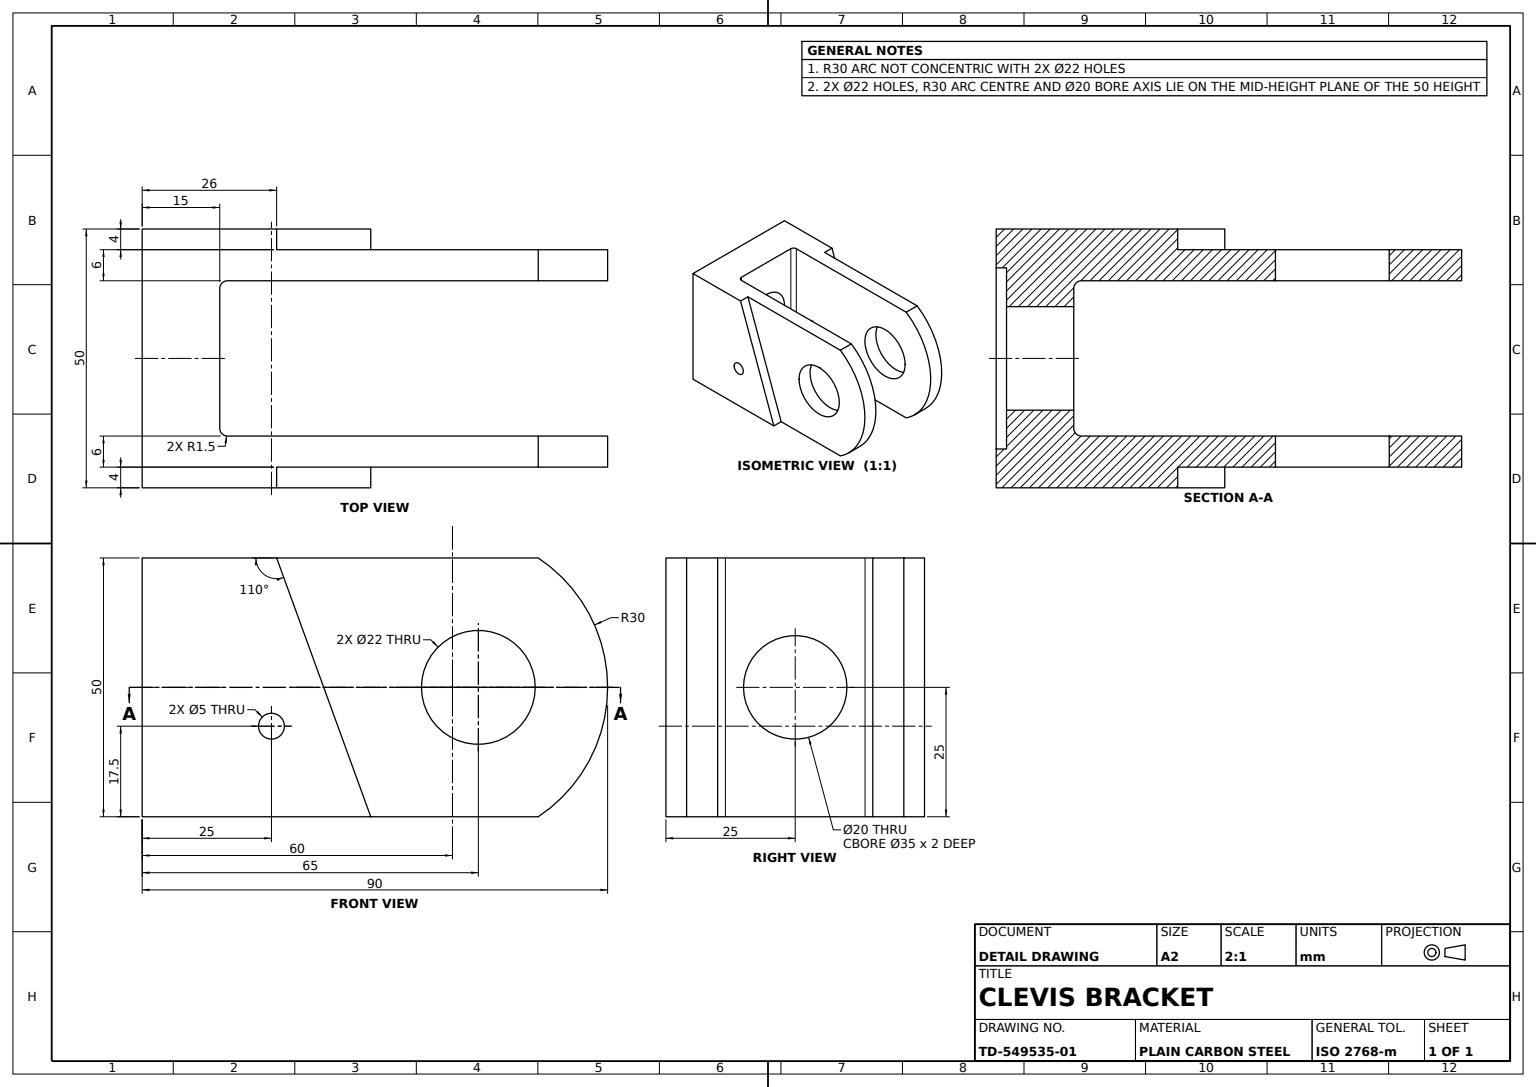
SolidWorks part; units mm, degrees
material "Plain Carbon Steel"
ref_plane "Front Plane" through (0, 0, 0) normal (0, 0, 1) x (1, 0, 0)
ref_plane "Top Plane" through (0, 0, 0) normal (0, 1, 0) x (1, 0, 0)
ref_plane "Right Plane" through (0, 0, 0) normal (1, 0, 0) x (0, 0, -1)
sketch "Clevis Body Profile" plane through (0, 0, 0) normal (0, 0, 1) x (1, 0, 0)
  line L0 (-65, 25) -> (11.5831, 25)
  line L1 (-65, 25) -> (-65, -25)
  line L2 (-65, -25) -> (11.5831, -25)
  circle A0 centre (0, 0) radius 11
  arc A2 (11.5831, 25) -> (11.5831, -25) centre (-5, 0) cw
  circle A3 centre (-40, -7.5) radius 2.5
  point P5 (25, 0)
  dimension "D1" = 22
  dimension "D2" = 90
  dimension "D3" = 30
  dimension "D6" = 5
  dimension "D4" = 50
  dimension "D5" = 65
  dimension "D7" = 17.5
  dimension "D8" = 25
extrude "Clevis Body" add sketch "Clevis Body Profile" along normal mid plane 50
sketch "Clevis Slot Sketch" plane through (0, 25, 0) normal (0, 1, 0) x (1, 0, 0)
  line L1 (-50, 15) -> (40.5323, 15)
  line L2 (-50, 15) -> (-50, -15)
  line L3 (-50, -15) -> (40.5323, -15)
  line L4 (40.5323, 15) -> (40.5323, -15)
  line L5 (-65, -25) -> (-65, 25) construction
  point P4 (-50, 0)
  dimension "D1" = 30
  dimension "D2" = 15
  dimension "D3" = 105.5323
extrude "Clevis Slot 30mm" cut sketch "Clevis Slot Sketch" against normal through all
sketch "Ear Side Relief Sketch" plane through (0, 0, 25) normal (0, 0, 1) x (1, 0, 0)
  line L0 (-39, 25) -> (-20.8015, -25)
  line L1 (11.5831, 25) -> (-65, 25) construction
  line L2 (-65, -25) -> (11.5831, -25) construction
  line L3 (-20.8015, -25) -> (11.5831, -25)
  line L4 (11.5831, 25) -> (-39, 25)
  line L5 (-65, 25) -> (-65, -25) construction
  arc A0 (11.5831, -25) -> (11.5831, 25) centre (-5, 0) ccw construction
  arc A1 (11.5831, -25) -> (11.5831, 25) centre (-5, 0) ccw
  dimension "D1" = 26
  dimension "D2" = 110
extrude "Ear Side Relief" cut sketch "Ear Side Relief Sketch" against normal blind 4
mirror "Ear Side Relief Mirror" about plane through (0, 0, 0) normal (0, 0, 1) of "Ear Side Relief"
fillet "Slot Fillet R1.5" radius 1.5 2 edges at (-50, 0, 15) (-50, 0, -15)
hole_wizard "Pin Bore Ø20 CBore Ø35" positions "3DSketch1" profile "Sketch4" legacy
sketch3d "3DSketch1"
  point P0 (0, 0, 0)
  point P3 (-65, 0, 0)
sketch "Sketch4" plane through (-65, 0, 0) normal (0, 1, 0) x (0, 0, 1)
  line L0 (0, 0) -> (0, 99.7184)
  line L1 (0, 99.7184) -> (10, 99.7184)
  line L2 (10, 99.7184) -> (10, 2)
  line L3 (10, 2) -> (17.5, 2)
  line L4 (17.5, 2) -> (17.5, 0)
  line L5 (17.5, 0) -> (0, 0)
  line L6 (0, 110) -> (0, -10) construction
  dimension "Diameter" = 20
  dimension "Depth" = 100
  dimension "C-Bore Diameter" = 35
  dimension "C-Bore Depth" = 2
